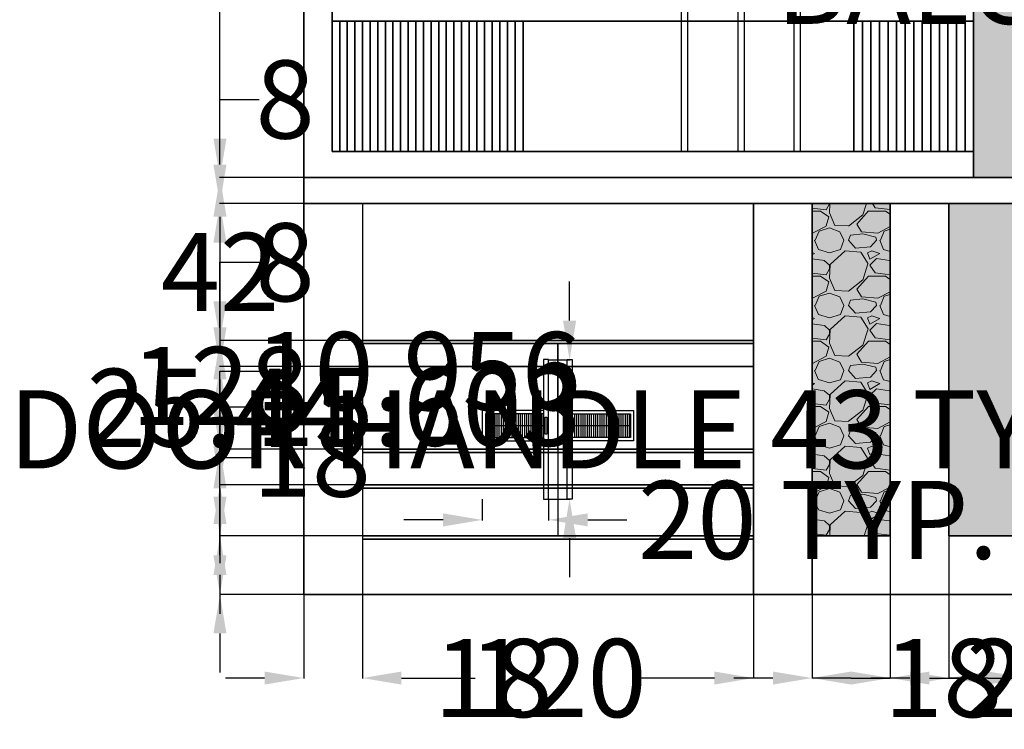
# Model space of a CAD drawing. Units: inches. Extents: x 172 to 828, y 190 to 777.
# Tile 1 of 9: x 172 to 474, y 190 to 408. Entities that reach past the tile are written whole.
import ezdxf

# ---------------------------------------------------------------- set-up
doc = ezdxf.new("R2010")
doc.units = ezdxf.units.IN
doc.header["$MEASUREMENT"] = 0
for name, color, linetype, lineweight in [('A-ANNO-DIMS', 2, 'Continuous', 18), ('A-DOOR', 4, 'Continuous', 25), ('A-ELEV', 7, 'Continuous', 35), ('A-ELEV-PATT', 8, 'Continuous', 13)]:
    doc.layers.add(name, color=color, linetype=linetype, lineweight=lineweight)
doc.styles.get("Standard").update_dxf_attribs({"font": 'arial.ttf'})
doc.dimstyles.get("Standard").update_dxf_attribs({"dimtxt": 24, "dimasz": 12, "dimexe": 0.18, "dimexo": 0.0625, "dimgap": 0.09, "dimtad": 0, "dimtih": 1, "dimtoh": 1, "dimdec": 0, "dimzin": 0, "dimdsep": 46, "dimlunit": 3, "dimtxsty": 'Standard', "dimcen": 0.09, "dimadec": 0, "dimazin": 0, "dimtfac": 1, "dimtdec": 0, "dimtofl": 0, "dimtmove": 0, "dimatfit": 3, "dimfxl": 1, "dimtolj": 1, "dimtzin": 0, "dimarcsym": 0})
pattern_1 = [(228.012788, (0.72, 1), (-8, -9), [0.134536, -13.319088]), (184.969741, (0.63, 0.9), (12, 1), [0.230868, -22.8559248]), (132.510447, (0.4, 0.88), (10, -11), [0.162788, -16.1160326]), (267.273689, (0.01, 0.63), (1, 20), [0.210238, -20.813558]), (292.833654, (0, 0.42), (-5, 12), [0.206155, -20.4093731]), (357.273689, (0.08, 0.23), (-20, 1), [0.210238, -20.813558]), (37.6942405, (0.29, 0.22), (-13, -10), [0.278029, -27.5248485]), (72.2553284, (0.51, 0.39), (7, 22), [0.262488, -25.9863215]), (121.4295656, (0.59, 0.64), (-8, 13), [0.21095, -20.8840731]), (175.236358, (0.48, 0.82), (11, -1), [0.240832, -11.8007626]), (222.397438, (0.24, 0.84), (-12, -11), [0.311448, -30.833375]), (138.814075, (1, 0.62), (-7, 6), [0.106301, -10.5238448]), (171.4692344, (0.92, 0.69), (13, -2), [0.202237, -20.0215114]), (225, (0.72, 0.72), (-1e-16, -1), [0.141421, -1.2727926]), (203.19859, (0.65, 0.84), (5, 2), [0.076158, -7.5396151]), (291.80141, (0.58, 0.81), (-1, 3), [0.107703, -5.2774618]), (30.963757, (0.62, 0.71), (3, 2), [0.174929, -5.6560229]), (161.56505, (0.77, 0.8), (2, -1), [0.126491, -3.0357867]), (16.38954, (0, 0.81), (10, 3), [0.1772, -17.5428451]), (70.346176, (0.17, 0.86), (-4, -11), [0.148661, -14.7174077]), (293.19859, (0.77, 1), (-2, 5), [0.152315, -7.4634581]), (343.61046, (0.83, 0.86), (-10, 3), [0.1772, -17.5428451]), (339.443955, (0, 0.19), (-5, 2), [0.17088, -8.3731237]), (294.775141, (0.16, 0.13), (-5, 11), [0.143178, -14.1746431]), (66.80141, (0.78, 0), (2, 5), [0.152315, -7.4634581]), (17.354025, (0.84, 0.14), (-13, -4), [0.167631, -16.5954236]), (69.443955, (0.29, 0), (-2, -5), [0.08544, -8.4585637]), (101.309932, (0.72, 0), (-1, 4), [0.05099, -5.0480295]), (165.963757, (0.71, 0.05), (3, -1), [0.206155, -3.9169506]), (186.009006, (0.51, 0.1), (10, 1), [0.19105, -18.9139232]), (303.690068, (0.62, 0.62), (-1, 2), [0.144222, -3.4613293]), (353.1572266, (0.7, 0.5), (17, -2), [0.251794, -24.9275626]), (60.945396, (0.95, 0.47), (-4, -7), [0.102956, -10.1926741]), (90, (1, 0.56), (-1, 1), [0.06, -0.94]), (120.256437, (0.49, 0.13), (4, -7), [0.138924, -13.75352]), (48.012788, (0.42, 0.25), (8, 9), [0.269072, -13.184552]), (0, (0.6, 0.45), (1, 1), [0.26, -0.74]), (325.3048465, (0.86, 0.45), (10, -7), [0.158114, -15.6532743]), (254.054604, (0.99, 0.36), (-1, -4), [0.145602, -7.1345079]), (207.6459754, (0.95, 0.22), (-19, -10), [0.237065, -23.4694742]), (175.426079, (0.74, 0.11), (-13, 1), [0.250799, -24.8290734])]

# ---------------------------------------------------------------- blocks, each defined once
blk = doc.blocks.new('DOOR-GLAZED-DBL')
for p, q in [((36.57, 84), (0, 84)), ((0, 0), (0, 84)), ((2, 0), (2, 82)), ((17.29, 82), (2, 82)), ((17.29, 82), (17.29, 0)), ((34.57, 82), (19.29, 82)), ((19.29, 82), (19.29, 0)), ((34.57, 0), (34.57, 82)), ((36.57, 0), (36.57, 84))]:
    blk.add_line(p, q)
blk = doc.blocks.new('DOOR-HANDLE')
for points in [[(20.41, 42.8), (18.83, 42.8), (18.83, 0), (20.41, 0)], [(18.83, 26.19), (1, 26.19), (1, 18.91), (18.83, 18.91)], [(19.35, 25.18), (19.82, 25.18), (19.82, 19.94), (19.35, 19.94)]]:
    blk.add_lwpolyline(points, close=True)
blk.add_lwpolyline([(18.83, 27.19), (0, 27.19), (0, 17.91), (18.83, 17.91)])
blk = doc.blocks.new('*D4')
at = {"layer": 'A-ANNO-DIMS', "color": 0, "lineweight": -2, "transparency": 16777216}
for p, q in [((601.02, 471.8), (617.1, 471.8)), ((616.92, 459.8), (616.92, 431.1)), ((616.92, 377.39), (616.92, 406.09)), ((601.02, 365.39), (617.1, 365.39))]:
    blk.add_line(p, q, dxfattribs=at)
at = {"layer": 'A-ANNO-DIMS', "color": 0, "transparency": 16777216}
for points in [[(614.92, 459.8), (618.92, 459.8), (616.92, 471.8)], [(614.92, 377.39), (618.92, 377.39), (616.92, 365.39)]]:
    blk.add_solid(points, dxfattribs=at)
at = {"layer": 'Defpoints', "color": 0, "transparency": 16777216}
for p in [(600.96, 471.8), (616.92, 471.8), (600.96, 365.39)]:
    blk.add_point(p, dxfattribs=at)
at = {"layer": 'A-ANNO-DIMS', "color": 0, "transparency": 16777216, "insert": (616.92, 418.6), "char_height": 24, "attachment_point": 5}
blk.add_mtext('\\A1;BALCONY WINDOW 106 TYP.', dxfattribs=at)
blk = doc.blocks.new('*D8')
at = {"layer": 'A-ANNO-DIMS', "color": 0, "lineweight": -2, "transparency": 16777216}
for p, q in [((340.36, 315.47), (340.36, 327.47)), ((334, 303.47), (340.54, 303.47)), ((334, 260.68), (340.54, 260.68)), ((340.36, 248.68), (340.36, 236.68))]:
    blk.add_line(p, q, dxfattribs=at)
at = {"layer": 'A-ANNO-DIMS', "color": 0, "transparency": 16777216}
for points in [[(338.36, 315.47), (342.36, 315.47), (340.36, 303.47)], [(338.36, 248.68), (342.36, 248.68), (340.36, 260.68)]]:
    blk.add_solid(points, dxfattribs=at)
at = {"layer": 'Defpoints', "color": 0, "transparency": 16777216}
for p in [(333.94, 303.47), (340.36, 303.47), (333.94, 260.68)]:
    blk.add_point(p, dxfattribs=at)
at = {"layer": 'A-ANNO-DIMS', "color": 0, "transparency": 16777216, "insert": (340.36, 282.08), "char_height": 24, "attachment_point": 5}
blk.add_mtext('\\A1;DOOR HANDLE 43 TYP.', dxfattribs=at)
blk = doc.blocks.new('*D9')
at = {"layer": 'A-ANNO-DIMS', "color": 0, "lineweight": -2, "transparency": 16777216}
for p, q in [((313.53, 260.62), (313.53, 254.08)), ((333.94, 260.62), (333.94, 254.08)), ((301.53, 254.26), (289.53, 254.26)), ((345.94, 254.26), (357.94, 254.26))]:
    blk.add_line(p, q, dxfattribs=at)
at = {"layer": 'A-ANNO-DIMS', "color": 0, "transparency": 16777216}
for points in [[(301.53, 256.26), (301.53, 252.26), (313.53, 254.26)], [(345.94, 256.26), (345.94, 252.26), (333.94, 254.26)]]:
    blk.add_solid(points, dxfattribs=at)
at = {"layer": 'Defpoints', "color": 0, "transparency": 16777216}
for p in [(313.53, 260.68), (333.94, 260.68), (333.94, 254.26)]:
    blk.add_point(p, dxfattribs=at)
at = {"layer": 'A-ANNO-DIMS', "color": 0, "transparency": 16777216, "insert": (416.65, 254.26), "char_height": 24, "attachment_point": 5}
blk.add_mtext('\\A1;20 TYP.', dxfattribs=at)
blk = doc.blocks.new('*D10')
at = {"layer": 'A-ANNO-DIMS', "color": 0, "lineweight": -2, "transparency": 16777216}
for p, q in [((258.78, 231.45), (258.78, 761.27)), ((270.78, 761.09), (412.23, 761.09)), ((606.78, 761.09), (465.33, 761.09)), ((618.78, 735.45), (618.78, 761.27))]:
    blk.add_line(p, q, dxfattribs=at)
at = {"layer": 'A-ANNO-DIMS', "color": 0, "transparency": 16777216}
for points in [[(270.78, 763.09), (270.78, 759.09), (258.78, 761.09)], [(606.78, 763.09), (606.78, 759.09), (618.78, 761.09)]]:
    blk.add_solid(points, dxfattribs=at)
at = {"layer": 'Defpoints', "color": 0, "transparency": 16777216}
for p in [(618.78, 761.09), (618.78, 735.39), (258.78, 231.39)]:
    blk.add_point(p, dxfattribs=at)
at = {"layer": 'A-ANNO-DIMS', "color": 0, "transparency": 16777216, "insert": (438.78, 761.09), "char_height": 24, "attachment_point": 5}
blk.add_mtext('\\A1;360', dxfattribs=at)
blk = doc.blocks.new('*D12')
at = {"layer": 'A-ANNO-DIMS', "color": 0, "lineweight": -2, "transparency": 16777216}
for p, q in [((258.72, 359.39), (232.9, 359.39)), ((233.08, 347.39), (233.08, 307.74)), ((233.08, 243.39), (233.08, 283.05)), ((258.72, 231.39), (232.9, 231.39))]:
    blk.add_line(p, q, dxfattribs=at)
at = {"layer": 'A-ANNO-DIMS', "color": 0, "transparency": 16777216}
for points in [[(231.08, 347.39), (235.08, 347.39), (233.08, 359.39)], [(231.08, 243.39), (235.08, 243.39), (233.08, 231.39)]]:
    blk.add_solid(points, dxfattribs=at)
at = {"layer": 'Defpoints', "color": 0, "transparency": 16777216}
for p in [(233.08, 359.39), (258.78, 359.39), (258.78, 231.39)]:
    blk.add_point(p, dxfattribs=at)
at = {"layer": 'A-ANNO-DIMS', "color": 0, "transparency": 16777216, "insert": (233.08, 295.39), "char_height": 24, "attachment_point": 5}
blk.add_mtext('\\A1;128', dxfattribs=at)
blk = doc.blocks.new('*D13')
at = {"layer": 'A-ANNO-DIMS', "color": 0, "lineweight": -2, "transparency": 16777216}
for p, q in [((258.72, 487.39), (232.9, 487.39)), ((233.08, 475.39), (233.08, 435.74)), ((233.08, 371.39), (233.08, 411.05)), ((258.72, 359.39), (232.9, 359.39))]:
    blk.add_line(p, q, dxfattribs=at)
at = {"layer": 'A-ANNO-DIMS', "color": 0, "transparency": 16777216}
for points in [[(231.08, 475.39), (235.08, 475.39), (233.08, 487.39)], [(231.08, 371.39), (235.08, 371.39), (233.08, 359.39)]]:
    blk.add_solid(points, dxfattribs=at)
at = {"layer": 'Defpoints', "color": 0, "transparency": 16777216}
for p in [(233.08, 487.39), (258.78, 487.39), (258.78, 359.39)]:
    blk.add_point(p, dxfattribs=at)
at = {"layer": 'A-ANNO-DIMS', "color": 0, "transparency": 16777216, "insert": (233.08, 423.39), "char_height": 24, "attachment_point": 5}
blk.add_mtext('\\A1;128', dxfattribs=at)
blk = doc.blocks.new('*D15')
at = {"layer": 'A-ANNO-DIMS', "color": 0, "lineweight": -2, "transparency": 16777216}
for p, q in [((233.08, 371.39), (233.08, 383.39)), ((233.08, 383.39), (245.08, 383.39)), ((258.72, 359.39), (232.9, 359.39)), ((258.72, 351.39), (232.9, 351.39)), ((233.08, 339.39), (233.08, 327.39))]:
    blk.add_line(p, q, dxfattribs=at)
at = {"layer": 'A-ANNO-DIMS', "color": 0, "transparency": 16777216}
for points in [[(231.08, 371.39), (235.08, 371.39), (233.08, 359.39)], [(231.08, 339.39), (235.08, 339.39), (233.08, 351.39)]]:
    blk.add_solid(points, dxfattribs=at)
at = {"layer": 'Defpoints', "color": 0, "transparency": 16777216}
for p in [(233.08, 359.39), (258.78, 359.39), (258.78, 351.39)]:
    blk.add_point(p, dxfattribs=at)
at = {"layer": 'A-ANNO-DIMS', "color": 0, "transparency": 16777216, "insert": (253.08, 383.39), "char_height": 24, "attachment_point": 5}
blk.add_mtext('\\A1;8', dxfattribs=at)
blk = doc.blocks.new('*D16')
at = {"layer": 'A-ANNO-DIMS', "color": 0, "lineweight": -2, "transparency": 16777216}
for p, q in [((258.78, 231.33), (258.78, 205.51)), ((276.78, 231.33), (276.78, 205.51)), ((246.78, 205.69), (234.78, 205.69)), ((288.78, 205.69), (300.78, 205.69))]:
    blk.add_line(p, q, dxfattribs=at)
at = {"layer": 'A-ANNO-DIMS', "color": 0, "transparency": 16777216}
for points in [[(246.78, 207.69), (246.78, 203.69), (258.78, 205.69)], [(288.78, 207.69), (288.78, 203.69), (276.78, 205.69)]]:
    blk.add_solid(points, dxfattribs=at)
at = {"layer": 'Defpoints', "color": 0, "transparency": 16777216}
for p in [(258.78, 231.39), (276.78, 231.39), (276.78, 205.69)]:
    blk.add_point(p, dxfattribs=at)
at = {"layer": 'A-ANNO-DIMS', "color": 0, "transparency": 16777216, "insert": (316.95, 205.69), "char_height": 24, "attachment_point": 5}
blk.add_mtext('\\A1;18', dxfattribs=at)
blk = doc.blocks.new('*D17')
at = {"layer": 'A-ANNO-DIMS', "color": 0, "lineweight": -2, "transparency": 16777216}
for p, q in [((276.78, 231.33), (276.78, 205.51)), ((396.78, 231.33), (396.78, 205.51)), ((288.78, 205.69), (311.35, 205.69)), ((384.78, 205.69), (362.21, 205.69))]:
    blk.add_line(p, q, dxfattribs=at)
at = {"layer": 'A-ANNO-DIMS', "color": 0, "transparency": 16777216}
for points in [[(288.78, 207.69), (288.78, 203.69), (276.78, 205.69)], [(384.78, 207.69), (384.78, 203.69), (396.78, 205.69)]]:
    blk.add_solid(points, dxfattribs=at)
at = {"layer": 'Defpoints', "color": 0, "transparency": 16777216}
for p in [(276.78, 231.39), (396.78, 231.39), (396.78, 205.69)]:
    blk.add_point(p, dxfattribs=at)
at = {"layer": 'A-ANNO-DIMS', "color": 0, "transparency": 16777216, "insert": (336.78, 205.69), "char_height": 24, "attachment_point": 5}
blk.add_mtext('\\A1;120', dxfattribs=at)
blk = doc.blocks.new('*D18')
at = {"layer": 'A-ANNO-DIMS', "color": 0, "lineweight": -2, "transparency": 16777216}
for p, q in [((396.78, 231.33), (396.78, 205.51)), ((414.78, 231.33), (414.78, 205.51)), ((384.78, 205.69), (372.78, 205.69)), ((426.78, 205.69), (438.78, 205.69))]:
    blk.add_line(p, q, dxfattribs=at)
at = {"layer": 'A-ANNO-DIMS', "color": 0, "transparency": 16777216}
for points in [[(384.78, 207.69), (384.78, 203.69), (396.78, 205.69)], [(426.78, 207.69), (426.78, 203.69), (414.78, 205.69)]]:
    blk.add_solid(points, dxfattribs=at)
at = {"layer": 'Defpoints', "color": 0, "transparency": 16777216}
for p in [(396.78, 231.39), (414.78, 231.39), (414.78, 205.69)]:
    blk.add_point(p, dxfattribs=at)
at = {"layer": 'A-ANNO-DIMS', "color": 0, "transparency": 16777216, "insert": (454.95, 205.69), "char_height": 24, "attachment_point": 5}
blk.add_mtext('\\A1;18', dxfattribs=at)
blk = doc.blocks.new('*D19')
at = {"layer": 'A-ANNO-DIMS', "color": 0, "lineweight": -2, "transparency": 16777216}
for p, q in [((438.78, 249.33), (438.78, 205.51)), ((414.78, 231.33), (414.78, 205.51)), ((402.78, 205.69), (390.78, 205.69)), ((450.78, 205.69), (462.78, 205.69))]:
    blk.add_line(p, q, dxfattribs=at)
at = {"layer": 'A-ANNO-DIMS', "color": 0, "transparency": 16777216}
for points in [[(402.78, 207.69), (402.78, 203.69), (414.78, 205.69)], [(450.78, 207.69), (450.78, 203.69), (438.78, 205.69)]]:
    blk.add_solid(points, dxfattribs=at)
at = {"layer": 'Defpoints', "color": 0, "transparency": 16777216}
for p in [(438.78, 249.39), (414.78, 231.39), (438.78, 205.69)]:
    blk.add_point(p, dxfattribs=at)
at = {"layer": 'A-ANNO-DIMS', "color": 0, "transparency": 16777216, "insert": (480.21, 205.69), "char_height": 24, "attachment_point": 5}
blk.add_mtext('\\A1;24', dxfattribs=at)
blk = doc.blocks.new('*D20')
at = {"layer": 'A-ANNO-DIMS', "color": 0, "lineweight": -2, "transparency": 16777216}
for p, q in [((438.78, 249.33), (438.78, 205.51)), ((456.78, 249.33), (456.78, 205.51)), ((426.78, 205.69), (414.78, 205.69)), ((468.78, 205.69), (480.78, 205.69))]:
    blk.add_line(p, q, dxfattribs=at)
at = {"layer": 'A-ANNO-DIMS', "color": 0, "transparency": 16777216}
for points in [[(426.78, 207.69), (426.78, 203.69), (438.78, 205.69)], [(468.78, 207.69), (468.78, 203.69), (456.78, 205.69)]]:
    blk.add_solid(points, dxfattribs=at)
at = {"layer": 'Defpoints', "color": 0, "transparency": 16777216}
for p in [(438.78, 249.39), (456.78, 249.39), (456.78, 205.69)]:
    blk.add_point(p, dxfattribs=at)
at = {"layer": 'A-ANNO-DIMS', "color": 0, "transparency": 16777216, "insert": (496.95, 205.69), "char_height": 24, "attachment_point": 5}
blk.add_mtext('\\A1;18', dxfattribs=at)
blk = doc.blocks.new('*D21')
at = {"layer": 'A-ANNO-DIMS', "color": 0, "lineweight": -2, "transparency": 16777216}
for p, q in [((456.78, 249.33), (456.78, 205.51)), ((480.78, 231.33), (480.78, 205.51)), ((444.78, 205.69), (432.78, 205.69)), ((492.78, 205.69), (504.78, 205.69))]:
    blk.add_line(p, q, dxfattribs=at)
at = {"layer": 'A-ANNO-DIMS', "color": 0, "transparency": 16777216}
for points in [[(444.78, 207.69), (444.78, 203.69), (456.78, 205.69)], [(492.78, 207.69), (492.78, 203.69), (480.78, 205.69)]]:
    blk.add_solid(points, dxfattribs=at)
at = {"layer": 'Defpoints', "color": 0, "transparency": 16777216}
for p in [(456.78, 249.39), (480.78, 231.39), (480.78, 205.69)]:
    blk.add_point(p, dxfattribs=at)
at = {"layer": 'A-ANNO-DIMS', "color": 0, "transparency": 16777216, "insert": (522.21, 205.69), "char_height": 24, "attachment_point": 5}
blk.add_mtext('\\A1;24', dxfattribs=at)
blk = doc.blocks.new('*D22')
at = {"layer": 'A-ANNO-DIMS', "color": 0, "lineweight": -2, "transparency": 16777216}
for p, q in [((480.78, 231.33), (480.78, 205.51)), ((498.78, 231.33), (498.78, 205.51)), ((468.78, 205.69), (456.78, 205.69)), ((510.78, 205.69), (522.78, 205.69))]:
    blk.add_line(p, q, dxfattribs=at)
at = {"layer": 'A-ANNO-DIMS', "color": 0, "transparency": 16777216}
for points in [[(468.78, 207.69), (468.78, 203.69), (480.78, 205.69)], [(510.78, 207.69), (510.78, 203.69), (498.78, 205.69)]]:
    blk.add_solid(points, dxfattribs=at)
at = {"layer": 'Defpoints', "color": 0, "transparency": 16777216}
for p in [(480.78, 231.39), (498.78, 231.39), (498.78, 205.69)]:
    blk.add_point(p, dxfattribs=at)
at = {"layer": 'A-ANNO-DIMS', "color": 0, "transparency": 16777216, "insert": (538.95, 205.69), "char_height": 24, "attachment_point": 5}
blk.add_mtext('\\A1;18', dxfattribs=at)
blk = doc.blocks.new('*D24')
at = {"layer": 'A-ANNO-DIMS', "color": 0, "lineweight": -2, "transparency": 16777216}
for p, q in [((233.08, 261.39), (233.08, 273.39)), ((233.08, 273.39), (245.08, 273.39)), ((276.72, 249.39), (232.9, 249.39)), ((276.72, 231.39), (232.9, 231.39)), ((233.08, 219.39), (233.08, 207.39))]:
    blk.add_line(p, q, dxfattribs=at)
at = {"layer": 'A-ANNO-DIMS', "color": 0, "transparency": 16777216}
for points in [[(231.08, 261.39), (235.08, 261.39), (233.08, 249.39)], [(231.08, 219.39), (235.08, 219.39), (233.08, 231.39)]]:
    blk.add_solid(points, dxfattribs=at)
at = {"layer": 'Defpoints', "color": 0, "transparency": 16777216}
for p in [(233.08, 249.39), (276.78, 249.39), (276.78, 231.39)]:
    blk.add_point(p, dxfattribs=at)
at = {"layer": 'A-ANNO-DIMS', "color": 0, "transparency": 16777216, "insert": (261.25, 273.39), "char_height": 24, "attachment_point": 5}
blk.add_mtext('\\A1;18', dxfattribs=at)
blk = doc.blocks.new('*D25')
at = {"layer": 'A-ANNO-DIMS', "color": 0, "lineweight": -2, "transparency": 16777216}
for p, q in [((233.08, 277), (233.08, 289)), ((233.08, 289), (245.08, 289)), ((276.72, 265), (232.9, 265)), ((276.72, 249.39), (232.9, 249.39)), ((233.08, 237.39), (233.08, 225.39))]:
    blk.add_line(p, q, dxfattribs=at)
at = {"layer": 'A-ANNO-DIMS', "color": 0, "transparency": 16777216}
for points in [[(231.08, 277), (235.08, 277), (233.08, 265)], [(231.08, 237.39), (235.08, 237.39), (233.08, 249.39)]]:
    blk.add_solid(points, dxfattribs=at)
at = {"layer": 'Defpoints', "color": 0, "transparency": 16777216}
for p in [(233.08, 265), (276.78, 265), (276.78, 249.39)]:
    blk.add_point(p, dxfattribs=at)
at = {"layer": 'A-ANNO-DIMS', "color": 0, "transparency": 16777216, "insert": (293.86, 289), "char_height": 24, "attachment_point": 5}
blk.add_mtext('\\A1;15.603', dxfattribs=at)
blk = doc.blocks.new('*D26')
at = {"layer": 'A-ANNO-DIMS', "color": 0, "lineweight": -2, "transparency": 16777216}
for p, q in [((233.08, 287.95), (233.08, 299.95)), ((233.08, 299.95), (245.08, 299.95)), ((396.72, 275.95), (232.9, 275.95)), ((396.72, 265), (232.9, 265)), ((233.08, 253), (233.08, 241))]:
    blk.add_line(p, q, dxfattribs=at)
at = {"layer": 'A-ANNO-DIMS', "color": 0, "transparency": 16777216}
for points in [[(231.08, 287.95), (235.08, 287.95), (233.08, 275.95)], [(231.08, 253), (235.08, 253), (233.08, 265)]]:
    blk.add_solid(points, dxfattribs=at)
at = {"layer": 'Defpoints', "color": 0, "transparency": 16777216}
for p in [(233.08, 275.95), (396.78, 275.95), (396.78, 265)]:
    blk.add_point(p, dxfattribs=at)
at = {"layer": 'A-ANNO-DIMS', "color": 0, "transparency": 16777216, "insert": (293.85, 299.95), "char_height": 24, "attachment_point": 5}
blk.add_mtext('\\A1;10.956', dxfattribs=at)
blk = doc.blocks.new('*D27')
at = {"layer": 'A-ANNO-DIMS', "color": 0, "lineweight": -2, "transparency": 16777216}
for p, q in [((233.08, 313.39), (233.08, 325.39)), ((276.72, 301.39), (232.9, 301.39)), ((276.72, 275.95), (232.9, 275.95)), ((233.08, 263.95), (233.08, 251.95))]:
    blk.add_line(p, q, dxfattribs=at)
at = {"layer": 'A-ANNO-DIMS', "color": 0, "transparency": 16777216}
for points in [[(231.08, 313.39), (235.08, 313.39), (233.08, 301.39)], [(231.08, 263.95), (235.08, 263.95), (233.08, 275.95)]]:
    blk.add_solid(points, dxfattribs=at)
at = {"layer": 'Defpoints', "color": 0, "transparency": 16777216}
for p in [(233.08, 301.39), (276.78, 301.39), (276.78, 275.95)]:
    blk.add_point(p, dxfattribs=at)
at = {"layer": 'A-ANNO-DIMS', "color": 0, "transparency": 16777216, "insert": (233.08, 288.67), "char_height": 24, "attachment_point": 5}
blk.add_mtext('\\A1;25.44', dxfattribs=at)
blk = doc.blocks.new('*D28')
at = {"layer": 'A-ANNO-DIMS', "color": 0, "lineweight": -2, "transparency": 16777216}
for p, q in [((233.08, 321.39), (233.08, 333.39)), ((233.08, 333.39), (245.08, 333.39)), ((276.72, 309.39), (232.9, 309.39)), ((276.72, 301.39), (232.9, 301.39)), ((233.08, 289.39), (233.08, 277.39))]:
    blk.add_line(p, q, dxfattribs=at)
at = {"layer": 'A-ANNO-DIMS', "color": 0, "transparency": 16777216}
for points in [[(231.08, 321.39), (235.08, 321.39), (233.08, 309.39)], [(231.08, 289.39), (235.08, 289.39), (233.08, 301.39)]]:
    blk.add_solid(points, dxfattribs=at)
at = {"layer": 'Defpoints', "color": 0, "transparency": 16777216}
for p in [(233.08, 309.39), (276.78, 309.39), (276.78, 301.39)]:
    blk.add_point(p, dxfattribs=at)
at = {"layer": 'A-ANNO-DIMS', "color": 0, "transparency": 16777216, "insert": (253.08, 333.39), "char_height": 24, "attachment_point": 5}
blk.add_mtext('\\A1;8', dxfattribs=at)
blk = doc.blocks.new('*D29')
at = {"layer": 'A-ANNO-DIMS', "color": 0, "lineweight": -2, "transparency": 16777216}
for p, q in [((233.079175, 363.392291), (233.079175, 375.392291)), ((276.716675, 351.392291), (232.899175, 351.392291)), ((276.716675, 309.392291), (232.899175, 309.392291)), ((233.079175, 297.392291), (233.079175, 285.392291))]:
    blk.add_line(p, q, dxfattribs=at)
at = {"layer": 'A-ANNO-DIMS', "color": 0, "transparency": 16777216}
for points in [[(231.079175, 363.392291), (235.079175, 363.392291), (233.079175, 351.392291)], [(231.079175, 297.392291), (235.079175, 297.392291), (233.079175, 309.392291)]]:
    blk.add_solid(points, dxfattribs=at)
at = {"layer": 'Defpoints', "color": 0, "transparency": 16777216}
for p in [(233.079175, 351.392291), (276.779175, 351.392291), (276.779175, 309.392291)]:
    blk.add_point(p, dxfattribs=at)
at = {"layer": 'A-ANNO-DIMS', "color": 0, "transparency": 16777216, "insert": (233.079175, 330.392291), "char_height": 24, "attachment_point": 5}
blk.add_mtext('\\A1;42', dxfattribs=at)

msp = doc.modelspace()

# ---------------------------------------------------------------- hatches: boundary and pattern name
at = {"layer": 'A-ELEV-PATT'}
h = msp.add_hatch(dxfattribs=at)
h.set_pattern_fill('GRAVEL', color=256)
h.set_pattern_definition(pattern_1)
h.paths.add_polyline_path([(438.7792, 351.3923), (414.7792, 351.3923), (414.7792, 249.3923), (438.7792, 249.3923)])
h.paths.add_polyline_path([(480.7792, 351.3923), (456.7792, 351.3923), (456.7792, 249.3923), (480.7792, 249.3923)])
h.paths.add_polyline_path([(488.4232, 479.3923), (472.3356, 479.3923), (472.3356, 359.3923), (488.4232, 359.3923)])
h.paths.add_polyline_path([(488.4232, 607.3923), (472.3356, 607.3923), (472.3356, 487.3923), (488.4232, 487.3923)])
h = msp.add_hatch(dxfattribs=at)
h.set_pattern_fill('GRAVEL', color=256)
h.set_pattern_definition(pattern_1)
h.paths.add_polyline_path([(480.7792, 351.3923), (456.7792, 351.3923), (456.7792, 249.3923), (480.7792, 249.3923)])
h.paths.add_polyline_path([(488.4232, 479.3923), (472.3356, 479.3923), (472.3356, 359.3923), (488.4232, 359.3923)])
h.paths.add_polyline_path([(488.4232, 607.3923), (472.3356, 607.3923), (472.3356, 487.3923), (488.4232, 487.3923)])
h = msp.add_hatch(dxfattribs=at)
h.set_pattern_fill('GRAVEL', color=256, scale=20)
h.set_pattern_definition([(228.01279, (14.4, 20), (-160, -180), [2.69072, -266.38176]), (184.96974, (12.6, 18), (240, 20), [4.61736, -457.1185]), (132.51045, (8, 17.6), (200, -220), [3.25576, -322.32065]), (267.27369, (0.2, 12.6), (20, 400), [4.20476, -416.27116]), (292.83365, (0, 8.4), (-100, 240), [4.1231, -408.18746]), (357.27369, (1.6, 4.6), (-400, 20), [4.20476, -416.27116]), (37.69424, (5.8, 4.4), (-260, -200), [5.56058, -550.49697]), (72.25533, (10.2, 7.8), (140, 440), [5.24976, -519.72643]), (121.42957, (11.8, 12.8), (-160, 260), [4.219, -417.68146]), (175.23636, (9.6, 16.4), (220, -20), [4.81664, -236.01525]), (222.39744, (4.8, 16.8), (-240, -220), [6.22896, -616.6675]), (138.81407, (20, 12.4), (-140, 120), [2.126, -210.4769]), (171.46923, (18.4, 13.8), (260, -40), [4.04474, -400.43023]), (225, (14.4, 14.4), (-2e-15, -20), [2.8284, -25.45585]), (203.1986, (13, 16.8), (100, 40), [1.52316, -150.7923]), (291.8014, (11.6, 16.2), (-20, 60), [2.15406, -105.54924]), (30.96376, (12.4, 14.2), (60, 40), [3.4986, -113.12046]), (161.56505, (15.4, 16), (40, -20), [2.5298, -60.71573]), (16.38954, (0, 16.2), (200, 60), [3.544, -350.8569]), (70.34618, (3.4, 17.2), (-80, -220), [2.97322, -294.34815]), (293.1986, (15.4, 20), (-40, 100), [3.0463, -149.26916]), (343.61046, (16.6, 17.2), (-200, 60), [3.544, -350.8569]), (339.44395, (0, 3.8), (-100, 40), [3.4176, -167.46247]), (294.77514, (3.2, 2.6), (-100, 220), [2.86356, -283.49286]), (66.8014, (15.6, 0), (40, 100), [3.0463, -149.26916]), (17.35402, (16.8, 2.8), (-260, -80), [3.35262, -331.90847]), (69.44395, (5.8, 0), (-40, -100), [1.7088, -169.17127]), (101.30993, (14.4, 0), (-20, 80), [1.0198, -100.9606]), (165.96376, (14.2, 1), (60, -20), [4.1231, -78.339]), (186.009, (10.2, 2), (200, 20), [3.821, -378.27846]), (303.6901, (12.4, 12.4), (-20, 40), [2.88444, -69.2266]), (353.15723, (14, 10), (340, -40), [5.03588, -498.55125]), (60.9454, (19, 9.4), (-80, -140), [2.0591, -203.8535]), (90, (20, 11.2), (-20, 20), [1.2, -18.8]), (120.25644, (9.8, 2.6), (80, -140), [2.77848, -275.0704]), (48.01279, (8.4, 5), (160, 180), [5.38144, -263.69104]), (0, (12, 9), (20, 20), [5.2, -14.8]), (325.30485, (17.2, 9), (200, -140), [3.16228, -313.0655]), (254.0546, (19.8, 7.2), (-20, -80), [2.91204, -142.69016]), (207.64598, (19, 4.4), (-380, -200), [4.7413, -469.38948]), (175.42608, (14.8, 2.2), (-260, 20), [5.01598, -496.58147])])
h.paths.add_polyline_path([(480.7792, 351.3923), (456.7792, 351.3923), (456.7792, 249.3923), (480.7792, 249.3923)])
h.paths.add_polyline_path([(472.3356, 479.3923), (464.3356, 479.3923), (464.3356, 359.3923), (472.3356, 359.3923)])
h.paths.add_polyline_path([(488.4232, 479.3923), (472.3356, 479.3923), (472.3356, 359.3923), (488.4232, 359.3923)])
h.paths.add_polyline_path([(472.3356, 607.3923), (464.3356, 607.3923), (464.3356, 487.3923), (472.3356, 487.3923)])
h.paths.add_polyline_path([(488.4232, 607.3923), (472.3356, 607.3923), (472.3356, 487.3923), (488.4232, 487.3923)])
h = msp.add_hatch(dxfattribs=at)
h.set_pattern_fill('GRAVEL', color=256, scale=20)
h.paths.add_polyline_path([(438.7792, 351.3923), (414.7792, 351.3923), (414.7792, 249.3923), (438.7792, 249.3923)])

# ---------------------------------------------------------------- linework, layer by layer
at = {"layer": 'A-DOOR'}
for p, q in [((276.7792, 351.3923), (276.7792, 231.3923)), ((336.7792, 275.9511), (336.7792, 308.3923)), ((336.7792, 308.3923), (336.7792, 249.3923)), ((314.7785, 286.8649), (314.7785, 279.5908)), ((315.4298, 286.8649), (315.4298, 279.5908)), ((316.0811, 286.8649), (316.0811, 279.5908)), ((316.7325, 286.8649), (316.7325, 279.5908)), ((317.3838, 286.8649), (317.3838, 279.5908)), ((318.0351, 286.8649), (318.0351, 279.5908)), ((318.6864, 286.8649), (318.6864, 279.5908)), ((319.3378, 286.8649), (319.3378, 279.5908)), ((319.9891, 286.8649), (319.9891, 279.5908)), ((320.6404, 286.8649), (320.6404, 279.5908)), ((321.2918, 286.8649), (321.2918, 279.5908)), ((321.9431, 286.8649), (321.9431, 279.5908)), ((322.5944, 286.8649), (322.5944, 279.5908)), ((323.2457, 286.8649), (323.2457, 279.5908)), ((323.8971, 286.8649), (323.8971, 279.5908)), ((324.5484, 286.8649), (324.5484, 279.5908)), ((325.1997, 286.8649), (325.1997, 279.5908)), ((325.851, 286.8649), (325.851, 279.5908)), ((326.5024, 286.8649), (326.5024, 279.5908)), ((327.1537, 286.8649), (327.1537, 279.5908)), ((327.805, 286.8649), (327.805, 279.5908)), ((328.4563, 286.8649), (328.4563, 279.5908)), ((329.1077, 286.8649), (329.1077, 279.5908)), ((329.759, 286.8649), (329.759, 279.5908)), ((330.4103, 286.8649), (330.4103, 279.5908)), ((331.0617, 286.8649), (331.0617, 279.5908)), ((331.713, 286.8649), (331.713, 279.5908)), ((332.3643, 286.8649), (332.3643, 279.5908)), ((341.194, 286.8649), (341.194, 279.5908)), ((341.8414, 286.8649), (341.8414, 279.5908)), ((342.4888, 286.8649), (342.4888, 279.5908)), ((343.1362, 286.8649), (343.1362, 279.5908)), ((343.7835, 286.8649), (343.7835, 279.5908)), ((344.4309, 286.8649), (344.4309, 279.5908)), ((345.0783, 286.8649), (345.0783, 279.5908)), ((345.7256, 286.8649), (345.7256, 279.5908)), ((346.373, 286.8649), (346.373, 279.5908)), ((347.0204, 286.8649), (347.0204, 279.5908)), ((347.6678, 286.8649), (347.6678, 279.5908)), ((348.3151, 286.8649), (348.3151, 279.5908)), ((348.9625, 286.8649), (348.9625, 279.5908)), ((349.6099, 286.8649), (349.6099, 279.5908)), ((350.2573, 286.8649), (350.2573, 279.5908)), ((350.9046, 286.8649), (350.9046, 279.5908)), ((351.552, 286.8649), (351.552, 279.5908)), ((352.1994, 286.8649), (352.1994, 279.5908)), ((352.8467, 286.8649), (352.8467, 279.5908)), ((353.4941, 286.8649), (353.4941, 279.5908)), ((354.1415, 286.8649), (354.1415, 279.5908)), ((354.7889, 286.8649), (354.7889, 279.5908)), ((355.4362, 286.8649), (355.4362, 279.5908)), ((356.0836, 286.8649), (356.0836, 279.5908)), ((356.731, 286.8649), (356.731, 279.5908)), ((357.3783, 286.8649), (357.3783, 279.5908)), ((358.0257, 286.8649), (358.0257, 279.5908)), ((358.6731, 286.8649), (358.6731, 279.5908)), ((314.5333, 283.2279), (332.3643, 283.2279)), ((341.194, 283.2279), (359.0251, 283.2279))]:
    msp.add_line(p, q, dxfattribs=at)
at = {"layer": 'A-ELEV'}
for p, q in [((258.7792, 487.3923), (258.7792, 359.3923)), ((258.7792, 359.3923), (258.7792, 479.3923)), ((267.4822, 367.3923), (267.4822, 479.3923)), ((464.3356, 479.3923), (464.3356, 359.3923)), ((464.3356, 407.3923), (267.4822, 407.3923)), ((269.8186, 367.3923), (269.8186, 407.3923)), ((272.155, 367.3923), (272.155, 407.3923)), ((274.4914, 367.3923), (274.4914, 407.3923)), ((276.8278, 367.3923), (276.8278, 407.3923)), ((279.1642, 367.3923), (279.1642, 407.3923)), ((281.5006, 367.3923), (281.5006, 407.3923)), ((283.837, 367.3923), (283.837, 407.3923)), ((286.1735, 367.3923), (286.1735, 407.3923)), ((288.5099, 367.3923), (288.5099, 407.3923)), ((290.8463, 367.3923), (290.8463, 407.3923)), ((293.1827, 367.3923), (293.1827, 407.3923)), ((295.5191, 367.3923), (295.5191, 407.3923)), ((297.8555, 367.3923), (297.8555, 407.3923)), ((300.1919, 367.3923), (300.1919, 407.3923)), ((302.5283, 367.3923), (302.5283, 407.3923)), ((304.8647, 367.3923), (304.8647, 407.3923)), ((307.2011, 367.3923), (307.2011, 407.3923)), ((309.5375, 367.3923), (309.5375, 407.3923)), ((311.8739, 367.3923), (311.8739, 407.3923)), ((314.2715, 367.3923), (314.2715, 407.3923)), ((316.6079, 367.3923), (316.6079, 407.3923)), ((318.9443, 367.3923), (318.9443, 407.3923)), ((321.3419, 367.3923), (321.3419, 407.3923)), ((323.6783, 367.3923), (323.6783, 407.3923)), ((326.0759, 367.3923), (326.0759, 407.3923)), ((427.5926, 367.3923), (427.5926, 407.3923)), ((427.5926, 407.3923), (427.5926, 367.3923)), ((430.2171, 407.3923), (430.2171, 367.3923)), ((432.8416, 407.3923), (432.8416, 367.3923)), ((435.4661, 407.3923), (435.4661, 367.3923)), ((438.0906, 407.3923), (438.0906, 367.3923)), ((440.7151, 407.3923), (440.7151, 367.3923)), ((443.3396, 407.3923), (443.3396, 367.3923)), ((445.9641, 407.3923), (445.9641, 367.3923)), ((448.5886, 407.3923), (448.5886, 367.3923)), ((451.2131, 407.3923), (451.2131, 367.3923)), ((453.8376, 407.3923), (453.8376, 367.3923)), ((456.4621, 407.3923), (456.4621, 367.3923)), ((459.0866, 407.3923), (459.0866, 367.3923)), ((461.7111, 407.3923), (461.7111, 367.3923)), ((464.3356, 367.3923), (267.4822, 367.3923)), ((258.7792, 359.3923), (258.7792, 231.3923)), ((618.7792, 359.3923), (258.7792, 359.3923)), ((472.3356, 359.3923), (393.1206, 359.3923)), ((618.7792, 351.3923), (258.7792, 351.3923)), ((396.7792, 351.3923), (396.7792, 231.3923)), ((414.7792, 351.3923), (414.7792, 231.3923)), ((438.7792, 351.3923), (438.7792, 249.3923)), ((456.7792, 351.3923), (456.7792, 249.3923)), ((276.7792, 309.3923), (396.7792, 309.3923)), ((276.7792, 308.3923), (396.7792, 308.3923)), ((276.7792, 301.3923), (396.7792, 301.3923)), ((276.7792, 275.9511), (396.7792, 275.9511)), ((276.7792, 275.9511), (396.7792, 275.9511)), ((276.7792, 274.9511), (396.7792, 274.9511)), ((276.7792, 264.9953), (396.7792, 264.9953)), ((276.7792, 263.9953), (396.7792, 263.9953)), ((276.7792, 249.3923), (396.7792, 249.3923)), ((276.7792, 248.3923), (396.7792, 248.3923)), ((414.7792, 249.3923), (438.7792, 249.3923)), ((456.7792, 249.3923), (480.7792, 249.3923)), ((258.7792, 231.3923), (618.7792, 231.3923))]:
    msp.add_line(p, q, dxfattribs=at)

# ---------------------------------------------------------------- block references
at = {"layer": 'A-DOOR'}
for name, p in [('DOOR-GLAZED-DBL', (374.663, 367.392)), ('DOOR-HANDLE', (313.533, 260.678))]:
    msp.add_blockref(name, p, dxfattribs=at)
at = {"layer": 'A-DOOR', "extrusion": (0, 0, -1), "zscale": -1}
msp.add_blockref('DOOR-HANDLE', (-360.0254, 260.678), dxfattribs=at)

# ---------------------------------------------------------------- dimensions: what is measured, and where the dimension line sits
at = {"layer": 'A-ANNO-DIMS'}
for base, p1, p2, picture, middle in [((618.7792, 761.0923), (258.7792, 231.3923), (618.7792, 735.3923), '*D10', (438.7792, 761.0923)), ((438.7792, 205.6923), (414.7792, 231.3923), (438.7792, 249.3923), '*D19', (480.2143, 205.6923)), ((456.7792, 205.6923), (438.7792, 249.3923), (456.7792, 249.3923), '*D20', (496.9538, 205.6923)), ((480.7792, 205.6923), (456.7792, 249.3923), (480.7792, 231.3923), '*D21', (522.2143, 205.6923)), ((276.7792, 205.6923), (258.7792, 231.3923), (276.7792, 231.3923), '*D16', (316.9538, 205.6923)), ((396.7792, 205.6923), (276.7792, 231.3923), (396.7792, 231.3923), '*D17', (336.7792, 205.6923)), ((414.7792, 205.6923), (396.7792, 231.3923), (414.7792, 231.3923), '*D18', (454.9538, 205.6923)), ((498.7792, 205.6923), (480.7792, 231.3923), (498.7792, 231.3923), '*D22', (538.9538, 205.6923))]:
    dim = msp.add_linear_dim(base=base, p1=p1, p2=p2, dimstyle='Standard', override={"dimdec": 0, "dimlfac": 1, "dimrnd": 0, "dimzin": 0, "dimdsep": 46, "dimlunit": 2}, dxfattribs=at)
    dim.commit()
    dim.dimension.update_dxf_attribs({"geometry": picture, "text_midpoint": middle})
for base, p1, p2, text, picture, middle in [((616.9208, 471.8013), (600.9594, 365.3923), (600.9594, 471.8013), 'BALCONY WINDOW <> TYP.', '*D4', (616.9208, 418.5968)), ((340.3606, 303.4742), (333.9412, 260.6781), (333.9412, 303.4742), 'DOOR HANDLE <> TYP.', '*D8', (340.3606, 282.0761))]:
    dim = msp.add_linear_dim(base=base, p1=p1, p2=p2, angle=90, text=text, dimstyle='Standard', override={"dimdec": 0, "dimlfac": 1, "dimrnd": 0, "dimzin": 0, "dimdsep": 46, "dimlunit": 2}, dxfattribs=at)
    dim.commit()
    dim.dimension.update_dxf_attribs({"geometry": picture, "text_midpoint": middle})
for base, p1, p2, override, picture, middle in [((233.0792, 487.3923), (258.7792, 359.3923), (258.7792, 487.3923), {"dimdec": 0, "dimlfac": 1, "dimrnd": 0, "dimzin": 0, "dimdsep": 46, "dimlunit": 2}, '*D13', (233.0792, 423.3923)), ((233.0792, 359.3923), (258.7792, 351.3923), (258.7792, 359.3923), {"dimdec": 0, "dimlfac": 1, "dimrnd": 0, "dimzin": 0, "dimdsep": 46, "dimlunit": 2}, '*D15', (253.0764, 383.3923)), ((233.0792, 351.3923), (276.7792, 309.3923), (276.7792, 351.3923), {"dimdec": 0, "dimlfac": 1, "dimrnd": 0, "dimzin": 0, "dimdsep": 46, "dimlunit": 2}, '*D29', (233.0792, 330.3923)), ((233.0792, 359.3923), (258.7792, 231.3923), (258.7792, 359.3923), {"dimdec": 0, "dimlfac": 1, "dimrnd": 0, "dimzin": 0, "dimdsep": 46, "dimlunit": 2}, '*D12', (233.0792, 295.3923)), ((233.0792, 309.3923), (276.7792, 301.3923), (276.7792, 309.3923), {"dimdec": 0, "dimlfac": 1, "dimrnd": 0, "dimzin": 0, "dimdsep": 46, "dimlunit": 2}, '*D28', (253.0764, 333.3923)), ((233.0792, 301.3923), (276.7792, 275.9511), (276.7792, 301.3923), {"dimdec": 2, "dimlfac": 1, "dimrnd": 0, "dimzin": 0, "dimdsep": 46, "dimlunit": 2}, '*D27', (233.0792, 288.6717)), ((233.0792, 275.9511), (396.7792, 264.9953), (396.7792, 275.9511), {"dimdec": 3, "dimlfac": 1, "dimrnd": 0, "dimzin": 0, "dimdsep": 46, "dimlunit": 2}, '*D26', (293.8486, 299.9511)), ((233.0792, 264.9953), (276.7792, 249.3923), (276.7792, 264.9953), {"dimdec": 3, "dimlfac": 1, "dimrnd": 0, "dimzin": 0, "dimdsep": 46, "dimlunit": 2}, '*D25', (293.8568, 288.9953)), ((233.0792, 249.3923), (276.7792, 231.3923), (276.7792, 249.3923), {"dimdec": 0, "dimlfac": 1, "dimrnd": 0, "dimzin": 0, "dimdsep": 46, "dimlunit": 2}, '*D24', (261.2538, 273.3923))]:
    dim = msp.add_linear_dim(base=base, p1=p1, p2=p2, angle=90, dimstyle='Standard', override=override, dxfattribs=at)
    dim.commit()
    dim.dimension.update_dxf_attribs({"geometry": picture, "text_midpoint": middle})
dim = msp.add_linear_dim(base=(333.9412, 254.2587), p1=(313.5333, 260.6781), p2=(333.9412, 260.6781), text='<> TYP.', dimstyle='Standard', override={"dimdec": 0, "dimlfac": 1, "dimrnd": 0, "dimzin": 0, "dimdsep": 46, "dimlunit": 2}, dxfattribs=at)
dim.commit()
dim.dimension.update_dxf_attribs({"geometry": '*D9', "text_midpoint": (416.6479, 254.2587)})

doc.saveas('drawing.dxf')
